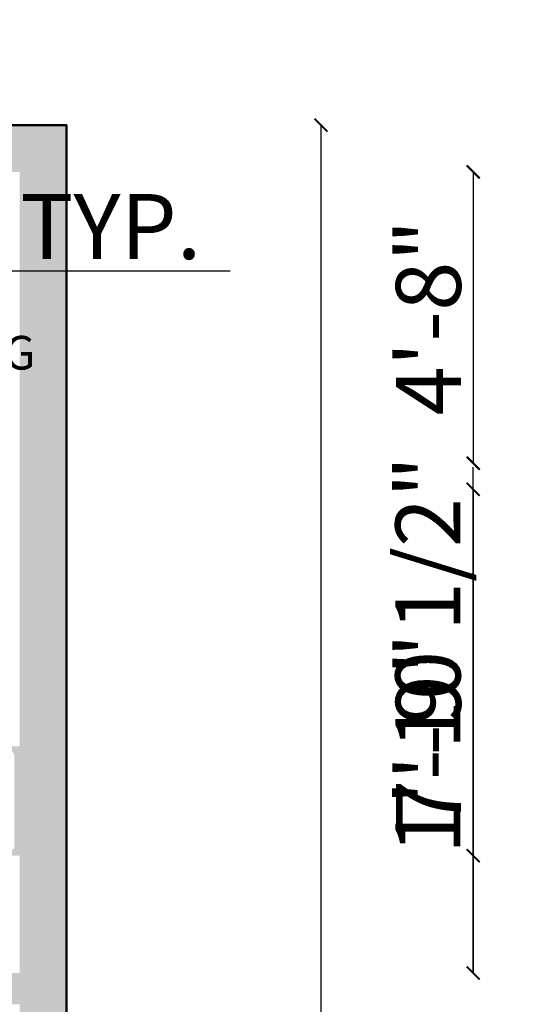
# Model space of a CAD drawing. Units: inches. Extents: x 2419 to 2878, y 1068 to 1713.
# Tile 19 of 20: x 2772 to 2870, y 1409 to 1598. Entities that reach past the tile are written whole.
import ezdxf

# ---------------------------------------------------------------- set-up
doc = ezdxf.new("R2010")
doc.units = ezdxf.units.IN
for name, color, linetype, lineweight in [('A-ANNO-DIMS', 2, 'Continuous', 18), ('A-AREA-IDEN', 7, 'Continuous', 18), ('A-FLOR-PRKG-PATT', 1, 'Continuous', 13), ('A-FURN-PATT', 254, 'Continuous', 13), ('A-WALL', 7, 'Continuous', 50)]:
    doc.layers.add(name, color=color, linetype=linetype, lineweight=lineweight)
doc.layers.add('A-FLOR-FIXT-PATT', color=254, linetype='Continuous', lineweight=13, true_color=0xd7ebd2)
doc.layers.add('A-WALL-PATT', color=18, linetype='Continuous', lineweight=13, true_color=0x000000)
doc.styles.get("Standard").update_dxf_attribs({"font": 'arial.ttf'})
doc.dimstyles.new('ISO-25', dxfattribs={"dimtxt": 12.5, "dimasz": 2.5, "dimexe": 1.25, "dimexo": 0.625, "dimtad": 1, "dimdec": 0, "dimlunit": 4, "dimtxsty": 'Standard', "dimblk": 'ARCHTICK', "dimcen": 2.5, "dimse1": 1, "dimse2": 1, "dimclrd": 4, "dimadec": 0, "dimazin": 0, "dimtfac": 1, "dimtdec": 0, "dimtmove": 0, "dimatfit": 3, "dimfxl": 1, "dimarcsym": 0})

# ---------------------------------------------------------------- blocks, each defined once
blk = doc.blocks.new('_ArchTick')
at = {"color": 0, "linetype": 'ByBlock', "const_width": 0.15}
blk.add_lwpolyline([(-0.5, -0.5), (0.5, 0.5)], dxfattribs=at)
blk = doc.blocks.new('*D16')
at = {"layer": 'A-ANNO-DIMS', "color": 0, "lineweight": -2, "transparency": 16777216}
blk.add_line((2471.51, 1623.24), (2780.51, 1623.24), dxfattribs=at)
at = {"layer": 'Defpoints', "color": 0, "transparency": 16777216}
for p in [(2780.51, 1623.24), (2471.51, 1577.81), (2780.51, 1577.81)]:
    blk.add_point(p, dxfattribs=at)
at = {"layer": 'A-ANNO-DIMS', "color": 0, "lineweight": -2, "transparency": 16777216, "xscale": 2.5, "yscale": 2.5, "zscale": 2.5, "rotation": 180}
blk.add_blockref('_ArchTick', (2471.51, 1623.24), dxfattribs=at)
at = {"layer": 'A-ANNO-DIMS', "color": 0, "lineweight": -2, "transparency": 16777216, "xscale": 2.5, "yscale": 2.5, "zscale": 2.5}
blk.add_blockref('_ArchTick', (2780.51, 1623.24), dxfattribs=at)
at = {"layer": 'A-ANNO-DIMS', "color": 0, "transparency": 16777216, "insert": (2626.01, 1630.25), "char_height": 12.5, "attachment_point": 5}
blk.add_mtext('25\'-9"', dxfattribs=at)
blk = doc.blocks.new('*D17')
at = {"layer": 'A-ANNO-DIMS', "color": 0, "lineweight": -2, "transparency": 16777216}
blk.add_line((2829.44, 1577.81), (2829.44, 1121.81), dxfattribs=at)
at = {"layer": 'Defpoints', "color": 0, "transparency": 16777216}
for p in [(2780.51, 1577.81), (2780.51, 1121.81), (2829.44, 1121.81)]:
    blk.add_point(p, dxfattribs=at)
at = {"layer": 'A-ANNO-DIMS', "color": 0, "lineweight": -2, "transparency": 16777216, "xscale": 2.5, "yscale": 2.5, "zscale": 2.5}
for p, rotation in [((2829.44, 1577.81), 90), ((2829.44, 1121.81), 270)]:
    blk.add_blockref('_ArchTick', p, dxfattribs=dict(at, rotation=rotation))
at = {"layer": 'A-ANNO-DIMS', "color": 0, "transparency": 16777216, "insert": (2822.42, 1349.81), "char_height": 12.5, "attachment_point": 5, "rotation": 90}
blk.add_mtext("38'", dxfattribs=at)
blk = doc.blocks.new('*D24')
at = {"layer": 'A-ANNO-DIMS', "color": 4, "lineweight": -2, "transparency": 16777216}
for p, q in [((2605.13, 1549.79), (2619.13, 1549.79)), ((2619.13, 1549.79), (2811.96, 1549.79))]:
    blk.add_line(p, q, dxfattribs=at)
at = {"layer": 'Defpoints', "color": 0, "transparency": 16777216}
for p in [(2605.13, 1551.89), (2619.13, 1551.89), (2619.13, 1549.79)]:
    blk.add_point(p, dxfattribs=at)
at = {"layer": 'A-ANNO-DIMS', "color": 4, "lineweight": -2, "transparency": 16777216, "xscale": 2.5, "yscale": 2.5, "zscale": 2.5, "rotation": 180}
blk.add_blockref('_ArchTick', (2605.13, 1549.79), dxfattribs=at)
at = {"layer": 'A-ANNO-DIMS', "color": 4, "lineweight": -2, "transparency": 16777216, "xscale": 2.5, "yscale": 2.5, "zscale": 2.5}
blk.add_blockref('_ArchTick', (2619.13, 1549.79), dxfattribs=at)
at = {"layer": 'A-ANNO-DIMS', "color": 0, "transparency": 16777216, "insert": (2716.8, 1556.69), "char_height": 12.5, "attachment_point": 5}
blk.add_mtext('TABLE LAMP 1\'-2" TYP.', dxfattribs=at)
blk = doc.blocks.new('*D37')
at = {"layer": 'A-ANNO-DIMS', "color": 4, "lineweight": -2, "transparency": 16777216}
for p, q in [((2736.32, 1605.01), (2771.51, 1605.01)), ((2771.51, 1605.01), (2818.42, 1605.01))]:
    blk.add_line(p, q, dxfattribs=at)
at = {"layer": 'Defpoints', "color": 0, "transparency": 16777216}
for p in [(2771.51, 1605.01), (2736.32, 1205.81), (2771.51, 1205.81)]:
    blk.add_point(p, dxfattribs=at)
at = {"layer": 'A-ANNO-DIMS', "color": 4, "lineweight": -2, "transparency": 16777216, "xscale": 2.5, "yscale": 2.5, "zscale": 2.5, "rotation": 180}
blk.add_blockref('_ArchTick', (2736.32, 1605.01), dxfattribs=at)
at = {"layer": 'A-ANNO-DIMS', "color": 4, "lineweight": -2, "transparency": 16777216, "xscale": 2.5, "yscale": 2.5, "zscale": 2.5}
blk.add_blockref('_ArchTick', (2771.51, 1605.01), dxfattribs=at)
at = {"layer": 'A-ANNO-DIMS', "color": 0, "transparency": 16777216, "insert": (2796.22, 1611.91), "char_height": 12.5, "attachment_point": 5}
blk.add_mtext('2\'-11"', dxfattribs=at)
blk = doc.blocks.new('*D49')
at = {"layer": 'A-ANNO-DIMS', "color": 4, "lineweight": -2, "transparency": 16777216}
for p, q in [((2732.27, 1605.01), (2750.85, 1605.01)), ((2750.85, 1605.01), (2815.78, 1605.01))]:
    blk.add_line(p, q, dxfattribs=at)
at = {"layer": 'Defpoints', "color": 0, "transparency": 16777216}
for p in [(2750.85, 1605.01), (2732.27, 1512.81), (2750.85, 1512.81)]:
    blk.add_point(p, dxfattribs=at)
at = {"layer": 'A-ANNO-DIMS', "color": 4, "lineweight": -2, "transparency": 16777216, "xscale": 2.5, "yscale": 2.5, "zscale": 2.5, "rotation": 180}
blk.add_blockref('_ArchTick', (2732.27, 1605.01), dxfattribs=at)
at = {"layer": 'A-ANNO-DIMS', "color": 4, "lineweight": -2, "transparency": 16777216, "xscale": 2.5, "yscale": 2.5, "zscale": 2.5}
blk.add_blockref('_ArchTick', (2750.85, 1605.01), dxfattribs=at)
at = {"layer": 'A-ANNO-DIMS', "color": 0, "transparency": 16777216, "insert": (2784.57, 1612.1), "char_height": 12.5, "attachment_point": 5}
blk.add_mtext('1\'-6 1/2"', dxfattribs=at)
blk = doc.blocks.new('*D51')
at = {"layer": 'A-ANNO-DIMS', "color": 4, "lineweight": -2, "transparency": 16777216}
for p, q in [((2738.51, 1079.92), (2771.51, 1079.92)), ((2771.51, 1079.92), (2808.71, 1079.92))]:
    blk.add_line(p, q, dxfattribs=at)
at = {"layer": 'Defpoints', "color": 0, "transparency": 16777216}
for p in [(2738.51, 1447.89), (2771.51, 1437.39), (2771.51, 1079.92)]:
    blk.add_point(p, dxfattribs=at)
at = {"layer": 'A-ANNO-DIMS', "color": 4, "lineweight": -2, "transparency": 16777216, "xscale": 2.5, "yscale": 2.5, "zscale": 2.5, "rotation": 180}
blk.add_blockref('_ArchTick', (2738.51, 1079.92), dxfattribs=at)
at = {"layer": 'A-ANNO-DIMS', "color": 4, "lineweight": -2, "transparency": 16777216, "xscale": 2.5, "yscale": 2.5, "zscale": 2.5}
blk.add_blockref('_ArchTick', (2771.51, 1079.92), dxfattribs=at)
at = {"layer": 'A-ANNO-DIMS', "color": 0, "transparency": 16777216, "insert": (2791.36, 1086.93), "char_height": 12.5, "attachment_point": 5}
blk.add_mtext('2\'-9"', dxfattribs=at)
blk = doc.blocks.new('*D52')
at = {"layer": 'A-ANNO-DIMS', "color": 4, "lineweight": -2, "transparency": 16777216}
for p, q in [((2858.71, 1437.39), (2858.71, 1512.03)), ((2858.71, 1414.81), (2858.71, 1437.39))]:
    blk.add_line(p, q, dxfattribs=at)
at = {"layer": 'Defpoints', "color": 0, "transparency": 16777216}
for p in [(2771.51, 1437.39), (2858.71, 1437.39), (2771.51, 1414.81)]:
    blk.add_point(p, dxfattribs=at)
at = {"layer": 'A-ANNO-DIMS', "color": 4, "lineweight": -2, "transparency": 16777216, "xscale": 2.5, "yscale": 2.5, "zscale": 2.5}
for p, rotation in [((2858.71, 1437.39), 90), ((2858.71, 1414.81), 270)]:
    blk.add_blockref('_ArchTick', p, dxfattribs=dict(at, rotation=rotation))
at = {"layer": 'A-ANNO-DIMS', "color": 0, "transparency": 16777216, "insert": (2851.63, 1475.96), "char_height": 12.5, "attachment_point": 5, "rotation": 90}
blk.add_mtext('1\'-10 1/2"', dxfattribs=at)
blk = doc.blocks.new('*D61')
at = {"layer": 'A-ANNO-DIMS', "color": 4, "lineweight": -2, "transparency": 16777216}
blk.add_line((2730.51, 1079.92), (2771.51, 1079.92), dxfattribs=at)
at = {"layer": 'Defpoints', "color": 0, "transparency": 16777216}
for p in [(2730.51, 1414.81), (2771.51, 1414.81), (2771.51, 1079.92)]:
    blk.add_point(p, dxfattribs=at)
at = {"layer": 'A-ANNO-DIMS', "color": 4, "lineweight": -2, "transparency": 16777216, "xscale": 2.5, "yscale": 2.5, "zscale": 2.5, "rotation": 180}
blk.add_blockref('_ArchTick', (2730.51, 1079.92), dxfattribs=at)
at = {"layer": 'A-ANNO-DIMS', "color": 4, "lineweight": -2, "transparency": 16777216, "xscale": 2.5, "yscale": 2.5, "zscale": 2.5}
blk.add_blockref('_ArchTick', (2771.51, 1079.92), dxfattribs=at)
at = {"layer": 'A-ANNO-DIMS', "color": 0, "transparency": 16777216, "insert": (2751.01, 1086.94), "char_height": 12.5, "attachment_point": 5}
blk.add_mtext('3\'-5"', dxfattribs=at)
blk = doc.blocks.new('*D62')
at = {"layer": 'A-ANNO-DIMS', "color": 4, "lineweight": -2, "transparency": 16777216}
blk.add_line((2858.71, 1507.81), (2858.71, 1414.81), dxfattribs=at)
at = {"layer": 'Defpoints', "color": 0, "transparency": 16777216}
for p in [(2771.51, 1507.81), (2771.51, 1414.81), (2858.71, 1414.81)]:
    blk.add_point(p, dxfattribs=at)
at = {"layer": 'A-ANNO-DIMS', "color": 4, "lineweight": -2, "transparency": 16777216, "xscale": 2.5, "yscale": 2.5, "zscale": 2.5}
for p, rotation in [((2858.71, 1507.81), 90), ((2858.71, 1414.81), 270)]:
    blk.add_blockref('_ArchTick', p, dxfattribs=dict(at, rotation=rotation))
at = {"layer": 'A-ANNO-DIMS', "color": 0, "transparency": 16777216, "insert": (2851.71, 1461.31), "char_height": 12.5, "attachment_point": 5, "rotation": 90}
blk.add_mtext('7\'-9"', dxfattribs=at)
blk = doc.blocks.new('*D63')
at = {"layer": 'A-ANNO-DIMS', "color": 4, "lineweight": -2, "transparency": 16777216}
blk.add_line((2858.71, 1568.81), (2858.71, 1512.81), dxfattribs=at)
at = {"layer": 'Defpoints', "color": 0, "transparency": 16777216}
for p in [(2771.51, 1568.81), (2771.51, 1512.81), (2858.71, 1512.81)]:
    blk.add_point(p, dxfattribs=at)
at = {"layer": 'A-ANNO-DIMS', "color": 4, "lineweight": -2, "transparency": 16777216, "xscale": 2.5, "yscale": 2.5, "zscale": 2.5}
for p, rotation in [((2858.71, 1568.81), 90), ((2858.71, 1512.81), 270)]:
    blk.add_blockref('_ArchTick', p, dxfattribs=dict(at, rotation=rotation))
at = {"layer": 'A-ANNO-DIMS', "color": 0, "transparency": 16777216, "insert": (2851.71, 1540.81), "char_height": 12.5, "attachment_point": 5, "rotation": 90}
blk.add_mtext('4\'-8"', dxfattribs=at)

msp = doc.modelspace()

# ---------------------------------------------------------------- hatches: boundary and pattern name
at = {"layer": 'A-FLOR-FIXT-PATT'}
h = msp.add_hatch(color=256, dxfattribs=at)
h.dxf.hatch_style = 1
h.paths.add_polyline_path([(2771.51, 1458.39), (2763.51, 1458.39), (2763.51, 1437.39), (2771.51, 1437.39)])
h.paths.add_polyline_path([(2770.51, 1456.39, 0.5), (2769.51, 1457.39), (2765.51, 1457.39, 0.5), (2764.51, 1456.39), (2764.51, 1439.39, 0.5), (2765.51, 1438.39), (2769.51, 1438.39, 0.5), (2770.51, 1439.39)], flags=16)
h.paths.add_polyline_path([(2706.38, 1408.81), (2685.38, 1408.81), (2685.38, 1400.81), (2706.38, 1400.81)])
h.paths.add_polyline_path([(2704.38, 1401.81, 0.5), (2705.38, 1402.81), (2705.38, 1406.81, 0.5), (2704.38, 1407.81), (2687.38, 1407.81, 0.5), (2686.38, 1406.81), (2686.38, 1402.81, 0.5), (2687.38, 1401.81)], flags=16)
h.paths.add_polyline_path([(2574.48, 1207.45), (2633.94, 1207.45), (2633.94, 1217.37), (2574.48, 1217.37)], flags=9)
h.paths.add_polyline_path([(2574.45, 1217.83), (2610.47, 1217.83), (2610.47, 1227.88), (2574.45, 1227.88)], flags=9)
h.paths.add_polyline_path([(2672.43, 1304.02), (2718.62, 1304.02), (2718.62, 1313.94), (2672.43, 1313.94)], flags=9)
h.paths.add_polyline_path([(2672.4, 1314.4), (2750.13, 1314.4), (2750.13, 1324.45), (2672.4, 1324.45)], flags=9)
h.paths.add_polyline_path([(2500.43, 1374.44), (2544.8, 1374.44), (2544.8, 1384.36), (2500.43, 1384.36)], flags=9)
h.paths.add_polyline_path([(2500.41, 1384.82), (2566.08, 1384.82), (2566.08, 1394.87), (2500.41, 1394.87)], flags=9)
h.paths.add_polyline_path([(2738.93, 1376.75), (2778.27, 1376.75), (2778.27, 1386.67), (2738.93, 1386.67)], flags=9)
h.paths.add_polyline_path([(2659.12, 1357.8), (2703.49, 1357.8), (2703.49, 1367.72), (2659.12, 1367.72)], flags=9)
h.paths.add_polyline_path([(2659.1, 1368.18), (2694.11, 1368.18), (2694.11, 1378.23), (2659.1, 1378.23)], flags=9)
h.paths.add_polyline_path([(2730.12, 1466.07), (2769.46, 1466.07), (2769.46, 1475.99), (2730.12, 1475.99)], flags=9)
h.paths.add_polyline_path([(2730.1, 1476.45), (2765.12, 1476.45), (2765.12, 1486.5), (2730.1, 1486.5)], flags=9)
h.paths.add_polyline_path([(2730.38, 1518.65), (2761.48, 1518.65), (2761.48, 1528.57), (2730.38, 1528.57)], flags=9)
h.paths.add_polyline_path([(2730.36, 1529.03), (2780.96, 1529.03), (2780.96, 1539.07), (2730.36, 1539.07)], flags=9)
h.paths.add_polyline_path([(2629.32, 1455.19), (2688.78, 1455.19), (2688.78, 1465.11), (2629.32, 1465.11)], flags=9)
h.paths.add_polyline_path([(2629.3, 1465.57), (2681.9, 1465.57), (2681.9, 1475.62), (2629.3, 1475.62)], flags=9)
h.paths.add_polyline_path([(2513.23, 1456.48), (2562.63, 1456.48), (2562.63, 1466.4), (2513.23, 1466.4)], flags=9)
h.paths.add_polyline_path([(2513.21, 1466.86), (2556.26, 1466.86), (2556.26, 1476.91), (2513.21, 1476.91)], flags=9)
h.paths.add_polyline_path([(2488.87, 1521.54), (2519.97, 1521.54), (2519.97, 1531.46), (2488.87, 1531.46)], flags=9)
h.paths.add_polyline_path([(2536.55, 1543.51), (2580.92, 1543.51), (2580.92, 1553.43), (2536.55, 1553.43)], flags=9)
h.paths.add_polyline_path([(2536.56, 1553.92), (2573.53, 1553.92), (2573.53, 1563.8), (2536.56, 1563.8)], flags=9)
at = {"layer": 'A-FLOR-PRKG-PATT'}
h = msp.add_hatch(color=256, dxfattribs=at)
h.dxf.hatch_style = 1
edge = h.paths.add_edge_path()
edge.add_ellipse((2561.37, 1279.45), major_axis=(3.99, 0), ratio=0.842304, start_angle=0.6466, end_angle=90)
edge.add_line((2561.37, 1282.81), (2511.57, 1282.81))
edge.add_ellipse((2511.57, 1279.45), major_axis=(3.99, 0), ratio=0.842304, start_angle=90, end_angle=179.3534)
edge.add_ellipse((10560.89, 1188.62), major_axis=(-8054.03, 0), ratio=0.8423039, start_angle=-0.646554, end_angle=-0.628237)
edge.add_ellipse((2509.23, 1276.91), major_axis=(1.69, 0), ratio=0.842304, start_angle=179.3718, end_angle=248.4648)
edge.add_ellipse((10560.33, 1188.62), major_axis=(8052.29, 0), ratio=0.8423039, start_angle=179.353446, end_angle=179.381357, ccw=False)
edge.add_ellipse((2511.01, 1279.45), major_axis=(2.25, 0), ratio=0.842304, start_angle=90, end_angle=179.3534, ccw=False)
edge.add_line((2511.01, 1281.35), (2561.94, 1281.35))
edge.add_ellipse((2561.94, 1279.45), major_axis=(-2.25, 0), ratio=0.842304, start_angle=180.6466, end_angle=270, ccw=False)
edge.add_ellipse((-5487.38, 1188.62), major_axis=(8052.29, 0), ratio=0.8423039, start_angle=0.528271, end_angle=0.646554, ccw=False)
edge.add_ellipse((2563.71, 1276.91), major_axis=(-1.69, 0), ratio=0.842304, start_angle=111.5352, end_angle=180.6282)
edge.add_ellipse((-5487.95, 1188.62), major_axis=(-8054.03, 0), ratio=0.8423039, start_angle=180.628237, end_angle=180.646554)
edge = h.paths.add_edge_path()
edge.add_ellipse((2564.91, 1261.91), major_axis=(-1.12, 0), ratio=0.842304, start_angle=180, end_angle=270)
edge.add_line((2564.91, 1262.86), (2564.43, 1262.86))
edge.add_ellipse((-5487.38, 1188.62), major_axis=(8052.29, 0), ratio=0.8423039, start_angle=0.383867, end_angle=0.528271, ccw=False)
edge.add_line((2564.65, 1242.56), (2564.91, 1242.56))
edge.add_ellipse((2564.91, 1243.51), major_axis=(-1.12, 0), ratio=0.842304, start_angle=90, end_angle=180)
edge.add_line((2566.03, 1243.51), (2566.03, 1261.91))
edge = h.paths.add_edge_path()
edge.add_ellipse((2564.91, 1174.99), major_axis=(1.12, 0), ratio=0.842304, start_angle=0, end_angle=90)
edge.add_line((2564.91, 1175.94), (2564.89, 1175.94))
edge.add_ellipse((-5487.38, 1188.62), major_axis=(8052.29, 0), ratio=0.8423039, start_angle=-0.134987, end_angle=-0.090229, ccw=False)
edge.add_ellipse((2163.34, 1170.91), major_axis=(401.54, 0), ratio=0.842304, start_angle=-2.18, end_angle=-0.1356, ccw=False)
edge.add_line((2564.47, 1155.64), (2564.91, 1155.64))
edge.add_ellipse((2564.91, 1156.59), major_axis=(-1.12, 0), ratio=0.842304, start_angle=90, end_angle=180)
edge.add_line((2566.03, 1156.59), (2566.03, 1174.99))
h.paths.add_polyline_path([(2574.48, 1207.45), (2633.94, 1207.45), (2633.94, 1217.37), (2574.48, 1217.37)], flags=9)
h.paths.add_polyline_path([(2574.45, 1217.83), (2610.47, 1217.83), (2610.47, 1227.88), (2574.45, 1227.88)], flags=9)
h.paths.add_polyline_path([(2672.43, 1304.02), (2718.62, 1304.02), (2718.62, 1313.94), (2672.43, 1313.94)], flags=9)
h.paths.add_polyline_path([(2672.4, 1314.4), (2750.13, 1314.4), (2750.13, 1324.45), (2672.4, 1324.45)], flags=9)
h.paths.add_polyline_path([(2500.43, 1374.44), (2544.8, 1374.44), (2544.8, 1384.36), (2500.43, 1384.36)], flags=9)
h.paths.add_polyline_path([(2500.41, 1384.82), (2566.08, 1384.82), (2566.08, 1394.87), (2500.41, 1394.87)], flags=9)
h.paths.add_polyline_path([(2738.93, 1376.75), (2778.27, 1376.75), (2778.27, 1386.67), (2738.93, 1386.67)], flags=9)
h.paths.add_polyline_path([(2659.12, 1357.8), (2703.49, 1357.8), (2703.49, 1367.72), (2659.12, 1367.72)], flags=9)
h.paths.add_polyline_path([(2659.1, 1368.18), (2694.11, 1368.18), (2694.11, 1378.23), (2659.1, 1378.23)], flags=9)
h.paths.add_polyline_path([(2730.12, 1466.07), (2769.46, 1466.07), (2769.46, 1475.99), (2730.12, 1475.99)], flags=9)
h.paths.add_polyline_path([(2730.1, 1476.45), (2765.12, 1476.45), (2765.12, 1486.5), (2730.1, 1486.5)], flags=9)
h.paths.add_polyline_path([(2730.38, 1518.65), (2761.48, 1518.65), (2761.48, 1528.57), (2730.38, 1528.57)], flags=9)
h.paths.add_polyline_path([(2730.36, 1529.03), (2780.96, 1529.03), (2780.96, 1539.07), (2730.36, 1539.07)], flags=9)
h.paths.add_polyline_path([(2629.32, 1455.19), (2688.78, 1455.19), (2688.78, 1465.11), (2629.32, 1465.11)], flags=9)
h.paths.add_polyline_path([(2629.3, 1465.57), (2681.9, 1465.57), (2681.9, 1475.62), (2629.3, 1475.62)], flags=9)
h.paths.add_polyline_path([(2513.23, 1456.48), (2562.63, 1456.48), (2562.63, 1466.4), (2513.23, 1466.4)], flags=9)
h.paths.add_polyline_path([(2513.21, 1466.86), (2556.26, 1466.86), (2556.26, 1476.91), (2513.21, 1476.91)], flags=9)
h.paths.add_polyline_path([(2488.87, 1521.54), (2519.97, 1521.54), (2519.97, 1531.46), (2488.87, 1531.46)], flags=9)
h.paths.add_polyline_path([(2536.55, 1543.51), (2580.92, 1543.51), (2580.92, 1553.43), (2536.55, 1553.43)], flags=9)
h.paths.add_polyline_path([(2536.56, 1553.92), (2573.53, 1553.92), (2573.53, 1563.8), (2536.56, 1563.8)], flags=9)
at = {"layer": 'A-FURN-PATT'}
h = msp.add_hatch(color=256, dxfattribs=at)
h.dxf.hatch_style = 1
h.paths.add_polyline_path([(2710.17, 1562.64), (2707.17, 1559.64), (2709.17, 1559.64, -0.414214), (2710.17, 1560.64)])
h.paths.add_polyline_path([(2711.17, 1559.64, 1), (2709.17, 1559.64, 1)])
h.paths.add_polyline_path([(2710.17, 1562.64), (2710.17, 1560.64, -0.414214), (2711.17, 1559.64), (2713.17, 1559.64)])
h.paths.add_polyline_path([(2713.17, 1559.64), (2711.17, 1559.64, -0.414214), (2710.17, 1558.64), (2710.17, 1556.64)])
h.paths.add_polyline_path([(2710.17, 1558.64, -0.414214), (2709.17, 1559.64), (2707.17, 1559.64), (2710.17, 1556.64)])
h.paths.add_polyline_path([(2613.13, 1558.89, 1), (2611.13, 1558.89, 1)])
h.paths.add_polyline_path([(2612.13, 1561.89), (2612.13, 1559.89, -0.414214), (2613.13, 1558.89), (2615.13, 1558.89)])
h.paths.add_polyline_path([(2612.13, 1559.89), (2612.13, 1561.89), (2609.13, 1558.89), (2611.13, 1558.89, -0.414214)])
h.paths.add_polyline_path([(2612.13, 1557.89, -0.414214), (2611.13, 1558.89), (2609.13, 1558.89), (2612.13, 1555.89)])
h.paths.add_polyline_path([(2574.48, 1207.45), (2633.94, 1207.45), (2633.94, 1217.37), (2574.48, 1217.37)], flags=9)
h.paths.add_polyline_path([(2574.45, 1217.83), (2610.47, 1217.83), (2610.47, 1227.88), (2574.45, 1227.88)], flags=9)
h.paths.add_polyline_path([(2672.43, 1304.02), (2718.62, 1304.02), (2718.62, 1313.94), (2672.43, 1313.94)], flags=9)
h.paths.add_polyline_path([(2672.4, 1314.4), (2750.13, 1314.4), (2750.13, 1324.45), (2672.4, 1324.45)], flags=9)
h.paths.add_polyline_path([(2500.43, 1374.44), (2544.8, 1374.44), (2544.8, 1384.36), (2500.43, 1384.36)], flags=9)
h.paths.add_polyline_path([(2500.41, 1384.82), (2566.08, 1384.82), (2566.08, 1394.87), (2500.41, 1394.87)], flags=9)
h.paths.add_polyline_path([(2738.93, 1376.75), (2778.27, 1376.75), (2778.27, 1386.67), (2738.93, 1386.67)], flags=9)
h.paths.add_polyline_path([(2659.12, 1357.8), (2703.49, 1357.8), (2703.49, 1367.72), (2659.12, 1367.72)], flags=9)
h.paths.add_polyline_path([(2659.1, 1368.18), (2694.11, 1368.18), (2694.11, 1378.23), (2659.1, 1378.23)], flags=9)
h.paths.add_polyline_path([(2730.12, 1466.07), (2769.46, 1466.07), (2769.46, 1475.99), (2730.12, 1475.99)], flags=9)
h.paths.add_polyline_path([(2730.1, 1476.45), (2765.12, 1476.45), (2765.12, 1486.5), (2730.1, 1486.5)], flags=9)
h.paths.add_polyline_path([(2730.38, 1518.65), (2761.48, 1518.65), (2761.48, 1528.57), (2730.38, 1528.57)], flags=9)
h.paths.add_polyline_path([(2730.36, 1529.03), (2780.96, 1529.03), (2780.96, 1539.07), (2730.36, 1539.07)], flags=9)
h.paths.add_polyline_path([(2629.32, 1455.19), (2688.78, 1455.19), (2688.78, 1465.11), (2629.32, 1465.11)], flags=9)
h.paths.add_polyline_path([(2629.3, 1465.57), (2681.9, 1465.57), (2681.9, 1475.62), (2629.3, 1475.62)], flags=9)
h.paths.add_polyline_path([(2513.23, 1456.48), (2562.63, 1456.48), (2562.63, 1466.4), (2513.23, 1466.4)], flags=9)
h.paths.add_polyline_path([(2513.21, 1466.86), (2556.26, 1466.86), (2556.26, 1476.91), (2513.21, 1476.91)], flags=9)
h.paths.add_polyline_path([(2488.87, 1521.54), (2519.97, 1521.54), (2519.97, 1531.46), (2488.87, 1531.46)], flags=9)
h.paths.add_polyline_path([(2536.55, 1543.51), (2580.92, 1543.51), (2580.92, 1553.43), (2536.55, 1553.43)], flags=9)
h.paths.add_polyline_path([(2536.56, 1553.92), (2573.53, 1553.92), (2573.53, 1563.8), (2536.56, 1563.8)], flags=9)
at = {"layer": 'A-WALL-PATT'}
h = msp.add_hatch(color=256, dxfattribs=at)
h.dxf.hatch_style = 1
h.paths.add_polyline_path([(2780.51, 1577.81), (2471.51, 1577.81), (2471.51, 1121.81), (2780.51, 1121.81)])
h.paths.add_polyline_path([(2480.51, 1568.81), (2771.51, 1568.81), (2771.51, 1130.81), (2480.51, 1130.81)], flags=16)
h.paths.add_polyline_path([(2528.51, 1568.81), (2528.51, 1512.81), (2594.51, 1512.81), (2594.51, 1414.81), (2596.57, 1414.81), (2596.57, 1441.61), (2597.82, 1441.61), (2597.82, 1441.58, -0.384016), (2625.03, 1414.81), (2725.51, 1414.81), (2725.51, 1567.55), (2728.3, 1567.55), (2746.89, 1567.55), (2746.89, 1566.73), (2746.87, 1566.73, -0.367216), (2730.51, 1549.09), (2730.51, 1512.81), (2750.85, 1512.81), (2750.85, 1510.03, -0.401453), (2733.08, 1491.46), (2733.08, 1491.44), (2732.27, 1491.44), (2732.27, 1507.81), (2730.51, 1507.81), (2730.51, 1408.81), (2736.51, 1408.81), (2736.51, 1349.81), (2632.51, 1349.81), (2632.51, 1408.81), (2528.51, 1408.81), (2528.51, 1414.81), (2503.97, 1414.81), (2503.97, 1494.85), (2558.38, 1494.85), (2558.38, 1507.81), (2529.96, 1507.81, -0.414214), (2530.82, 1506.96), (2530.82, 1497.26, -0.414214), (2529.96, 1496.4), (2514.56, 1496.4, -0.414214), (2513.7, 1497.26), (2513.7, 1506.96, -0.414214), (2514.56, 1507.81), (2528.51, 1507.81), (2528.51, 1512.81), (2480.51, 1512.81)], flags=0)
h.paths.add_polyline_path([(2516.26, 1507.81), (2528.26, 1507.81), (2528.26, 1505.81), (2523.42, 1505.81), (2524.07, 1504.67), (2529.39, 1504.67, -0.414214), (2529.96, 1504.1), (2529.96, 1497.83, -0.414214), (2529.39, 1497.26), (2515.13, 1497.26, -0.414214), (2514.56, 1497.83), (2514.56, 1504.1, -0.414214), (2515.13, 1504.67), (2520.69, 1504.67), (2521.34, 1505.81), (2516.26, 1505.81)], flags=0)
h.paths.add_polyline_path([(2522.02, 1505.53), (2522.82, 1507.32, -0.65506), (2522.25, 1506.06), (2522.19, 1505.93), (2522.43, 1505.53)], flags=0)
h.paths.add_polyline_path([(2522.83, 1500.97, -1), (2521.69, 1500.97, -1)], flags=0)
h.paths.add_polyline_path([(2522.55, 1500.97, -1), (2521.98, 1500.97, -1)], flags=0)
h.paths.add_polyline_path([(2482.01, 1470.63), (2499.89, 1470.63), (2499.89, 1448.27), (2482.01, 1448.27), (2482.01, 1452.74), (2481.26, 1452.74), (2481.26, 1449.76), (2480.51, 1449.76), (2480.51, 1469.14), (2481.26, 1469.14), (2481.26, 1466.16), (2482.01, 1466.16)], flags=0)
h.paths.add_polyline_path([(2488.71, 1466.16, -1), (2484.24, 1466.16, -1)], flags=0)
h.paths.add_polyline_path([(2496.17, 1466.16, -1), (2490.2, 1466.16, -1)], flags=0)
h.paths.add_polyline_path([(2487.97, 1466.16, -1), (2484.99, 1466.16, -1)], flags=0)
h.paths.add_polyline_path([(2495.42, 1466.16, -1), (2490.95, 1466.16, -1)], flags=0)
h.paths.add_polyline_path([(2487.22, 1466.16, -1), (2485.73, 1466.16, -1)], flags=0)
h.paths.add_polyline_path([(2494.68, 1466.16, -1), (2491.69, 1466.16, -1)], flags=0)
h.paths.add_polyline_path([(2499.11, 1468, -1), (2497.98, 1468, -1)], flags=0)
h.paths.add_polyline_path([(2493.93, 1466.16, -1), (2492.44, 1466.16, -1)], flags=0)
h.paths.add_polyline_path([(2499.37, 1463.71, -1), (2498.17, 1463.71, -1)], flags=0)
h.paths.add_polyline_path([(2484.24, 1461.69), (2496.17, 1461.69), (2496.17, 1457.22), (2484.24, 1457.22)], flags=0)
h.paths.add_polyline_path([(2484.99, 1460.94), (2495.42, 1460.94), (2495.42, 1457.96), (2484.99, 1457.96)], flags=0)
h.paths.add_polyline_path([(2586.88, 1510.03), (2587.69, 1510.03), (2587.69, 1491.44), (2586.88, 1491.44)], flags=0)
h.paths.add_polyline_path([(2499.26, 1459.41, -1), (2498.2, 1459.41, -1)], flags=0)
h.paths.add_polyline_path([(2489.46, 1452.74, -1), (2483.5, 1452.74, -1)], flags=0)
h.paths.add_polyline_path([(2557.3, 1408.81), (2557.3, 1413.09, -0.401453), (2584.57, 1441.58), (2584.57, 1441.61), (2585.82, 1441.61), (2585.82, 1413.09), (2585.82, 1408.81)], flags=0)
h.paths.add_polyline_path([(2488.71, 1452.74, -1), (2484.24, 1452.74, -1)], flags=0)
h.paths.add_polyline_path([(2495.42, 1452.74, -1), (2490.95, 1452.74, -1)], flags=0)
h.paths.add_polyline_path([(2487.97, 1452.74, -1), (2484.99, 1452.74, -1)], flags=0)
h.paths.add_polyline_path([(2494.68, 1452.74, -1), (2491.69, 1452.74, -1)], flags=0)
h.paths.add_polyline_path([(2487.22, 1452.74, -1), (2485.73, 1452.74, -1)], flags=0)
h.paths.add_polyline_path([(2499.18, 1454.44, -1), (2497.9, 1454.44, -1)], flags=0)
h.paths.add_polyline_path([(2493.93, 1452.74, -1), (2492.44, 1452.74, -1)], flags=0)
h.paths.add_polyline_path([(2499.3, 1450.64, -1), (2497.79, 1450.64, -1)], flags=0)
h.paths.add_polyline_path([(2619.13, 1558.89, -1), (2605.13, 1558.89, -1)], flags=0)
h.paths.add_polyline_path([(2609.13, 1558.89), (2612.13, 1561.89), (2615.13, 1558.89), (2612.13, 1555.89)], flags=0)
h.paths.add_polyline_path([(2611.13, 1558.89, -1), (2613.13, 1558.89, -1)], flags=0)
h.paths.add_polyline_path([(2633.68, 1568.81), (2693.68, 1568.81), (2693.68, 1488.81), (2633.68, 1488.81)], flags=0)
h.paths.add_polyline_path([(2641.68, 1554.41), (2641.68, 1567.61), (2662.48, 1567.61), (2662.48, 1554.41), (2664.88, 1554.41), (2664.88, 1567.61), (2685.68, 1567.61), (2685.68, 1552.41), (2680.48, 1552.41), (2693.68, 1539.21), (2678.48, 1539.21), (2678.48, 1554.41)], flags=0)
h.paths.add_polyline_path([(2637.51, 1408.81), (2731.51, 1408.81), (2731.51, 1354.81), (2637.51, 1354.81), (2637.51, 1357.98), (2635.3, 1357.98), (2635.3, 1358.79), (2637.51, 1358.79)], flags=0)
h.paths.add_polyline_path([(2717.17, 1559.64, -1), (2703.17, 1559.64, -1)], flags=0)
h.paths.add_polyline_path([(2707.17, 1559.64), (2710.17, 1562.64), (2713.17, 1559.64), (2710.17, 1556.64)], flags=0)
h.paths.add_polyline_path([(2709.17, 1559.64, -1), (2711.17, 1559.64, -1)], flags=0)
h.paths.add_polyline_path([(2685.38, 1408.81), (2706.38, 1408.81), (2706.38, 1400.81), (2699.88, 1400.81), (2701.88, 1394.81, -0.501323), (2696.92, 1375.95, -0.132891), (2694.83, 1375.95, -0.501317), (2689.88, 1394.81), (2691.88, 1400.81), (2688.88, 1400.81), (2688.88, 1399.31), (2685.88, 1399.31), (2685.88, 1400.31), (2687.88, 1400.31), (2687.88, 1400.81), (2685.38, 1400.81)], flags=0)
h.paths.add_polyline_path([(2687.38, 1407.81), (2704.38, 1407.81, -0.5), (2705.38, 1406.81), (2705.38, 1402.81, -0.5), (2704.38, 1401.81), (2687.38, 1401.81, -0.5), (2686.38, 1402.81), (2686.38, 1406.81, -0.5)], flags=0)
h.paths.add_polyline_path([(2639.51, 1205.81), (2634.51, 1205.81), (2634.51, 1293.81), (2637.51, 1293.81), (2639.51, 1293.81)], flags=0)
h.paths.add_polyline_path([(2691.88, 1394.81), (2699.88, 1394.81, -0.48008), (2697.52, 1377.29, -0.215004), (2694.23, 1377.29, -0.48008)], flags=0)
h.paths.add_polyline_path([(2757.51, 1453.89), (2763.51, 1451.89), (2763.51, 1454.89), (2762.01, 1454.89), (2762.01, 1457.89), (2763.01, 1457.89), (2763.01, 1455.89), (2763.51, 1455.89), (2763.51, 1458.39), (2771.51, 1458.39), (2771.51, 1437.39), (2763.51, 1437.39), (2763.51, 1443.89), (2757.51, 1441.89, -0.501323), (2738.65, 1446.85, -0.132891), (2738.65, 1448.94, -0.501317)], flags=0)
h.paths.add_polyline_path([(2739.99, 1449.54, -0.48008), (2757.51, 1451.89), (2757.51, 1443.89, -0.48008), (2739.99, 1446.25, -0.215004)], flags=0)
h.paths.add_polyline_path([(2765.51, 1457.39), (2769.51, 1457.39, -0.5), (2770.51, 1456.39), (2770.51, 1439.39, -0.5), (2769.51, 1438.39), (2765.51, 1438.39, -0.5), (2764.51, 1439.39), (2764.51, 1456.39, -0.5)], flags=0)
h = msp.add_hatch(color=256, dxfattribs=at)
h.dxf.hatch_style = 1
h.paths.add_polyline_path([(2771.51, 1354.81), (2736.51, 1354.81), (2736.51, 1408.81), (2771.51, 1408.81), (2771.51, 1414.81), (2625.03, 1414.81, -0.015108), (2625.09, 1413.09), (2625.09, 1408.81), (2632.51, 1408.81), (2632.51, 1376.56), (2635.3, 1376.56, -0.029838), (2637.51, 1376.43), (2637.51, 1408.81), (2731.51, 1408.81), (2731.51, 1354.81), (2637.51, 1354.81), (2637.51, 1357.98), (2635.3, 1357.98), (2632.51, 1357.98), (2632.51, 1349.81), (2771.51, 1349.81)])
h.paths.add_polyline_path([(2639.51, 1298.81), (2637.51, 1298.81), (2480.51, 1298.81), (2480.51, 1293.81), (2637.51, 1293.81), (2639.51, 1293.81)])
h.paths.add_polyline_path([(2639.51, 1293.81), (2637.51, 1293.81), (2634.51, 1293.81), (2634.51, 1244.65), (2638.79, 1244.65, -0.006332), (2639.51, 1244.64)])
h.paths.add_polyline_path([(2639.51, 1205.81), (2771.51, 1205.81), (2771.51, 1210.81), (2639.51, 1210.81), (2639.51, 1216.13), (2638.79, 1216.13), (2634.51, 1216.13), (2634.51, 1130.81), (2639.51, 1130.81)])
h.paths.add_polyline_path([(2596.57, 1413.09), (2596.57, 1414.81), (2585.82, 1414.81), (2585.82, 1413.09), (2585.82, 1408.81), (2596.57, 1408.81)])
h.paths.add_polyline_path([(2557.3, 1413.09, -0.015108), (2557.35, 1414.81), (2480.51, 1414.81), (2480.51, 1408.81), (2557.3, 1408.81)])
h.paths.add_polyline_path([(2574.48, 1207.45), (2633.94, 1207.45), (2633.94, 1217.37), (2574.48, 1217.37)], flags=9)
h.paths.add_polyline_path([(2574.45, 1217.83), (2610.47, 1217.83), (2610.47, 1227.88), (2574.45, 1227.88)], flags=9)
h.paths.add_polyline_path([(2672.43, 1304.02), (2718.62, 1304.02), (2718.62, 1313.94), (2672.43, 1313.94)], flags=9)
h.paths.add_polyline_path([(2672.4, 1314.4), (2750.13, 1314.4), (2750.13, 1324.45), (2672.4, 1324.45)], flags=9)
h.paths.add_polyline_path([(2500.43, 1374.44), (2544.8, 1374.44), (2544.8, 1384.36), (2500.43, 1384.36)], flags=9)
h.paths.add_polyline_path([(2500.41, 1384.82), (2566.08, 1384.82), (2566.08, 1394.87), (2500.41, 1394.87)], flags=9)
h.paths.add_polyline_path([(2738.93, 1376.75), (2778.27, 1376.75), (2778.27, 1386.67), (2738.93, 1386.67)], flags=9)
h.paths.add_polyline_path([(2659.12, 1357.8), (2703.49, 1357.8), (2703.49, 1367.72), (2659.12, 1367.72)], flags=25)
h.paths.add_polyline_path([(2659.1, 1368.18), (2694.11, 1368.18), (2694.11, 1378.23), (2659.1, 1378.23)], flags=25)
h.paths.add_polyline_path([(2730.12, 1466.07), (2769.46, 1466.07), (2769.46, 1475.99), (2730.12, 1475.99)], flags=9)
h.paths.add_polyline_path([(2730.1, 1476.45), (2765.12, 1476.45), (2765.12, 1486.5), (2730.1, 1486.5)], flags=9)
h.paths.add_polyline_path([(2730.38, 1518.65), (2761.48, 1518.65), (2761.48, 1528.57), (2730.38, 1528.57)], flags=9)
h.paths.add_polyline_path([(2730.36, 1529.03), (2780.96, 1529.03), (2780.96, 1539.07), (2730.36, 1539.07)], flags=9)
h.paths.add_polyline_path([(2629.32, 1455.19), (2688.78, 1455.19), (2688.78, 1465.11), (2629.32, 1465.11)], flags=9)
h.paths.add_polyline_path([(2629.3, 1465.57), (2681.9, 1465.57), (2681.9, 1475.62), (2629.3, 1475.62)], flags=9)
h.paths.add_polyline_path([(2513.23, 1456.48), (2562.63, 1456.48), (2562.63, 1466.4), (2513.23, 1466.4)], flags=9)
h.paths.add_polyline_path([(2513.21, 1466.86), (2556.26, 1466.86), (2556.26, 1476.91), (2513.21, 1476.91)], flags=9)
h.paths.add_polyline_path([(2488.87, 1521.54), (2519.97, 1521.54), (2519.97, 1531.46), (2488.87, 1531.46)], flags=9)
h.paths.add_polyline_path([(2536.55, 1543.51), (2580.92, 1543.51), (2580.92, 1553.43), (2536.55, 1553.43)], flags=9)
h.paths.add_polyline_path([(2536.56, 1553.92), (2573.53, 1553.92), (2573.53, 1563.8), (2536.56, 1563.8)], flags=9)

# ---------------------------------------------------------------- linework, layer by layer
at = {"layer": 'A-WALL'}
msp.add_lwpolyline([(2471.51, 1577.81), (2780.51, 1577.81), (2780.51, 1121.81), (2471.51, 1121.81)], close=True, dxfattribs=at)

# ---------------------------------------------------------------- texts
at = {"layer": 'A-AREA-IDEN'}
msp.add_text('DRESSING', height=6.475, dxfattribs=at).set_placement((2732.04, 1530.81))

# ---------------------------------------------------------------- dimensions: what is measured, and where the dimension line sits
at = {"layer": 'A-ANNO-DIMS'}
for base, p1, p2, override, picture, middle in [((2780.51, 1623.24), (2471.51, 1577.81), (2780.51, 1577.81), {"dimclrd": 0, "dimclre": 0, "dimclrt": 0}, '*D16', (2626.01, 1630.25)), ((2750.85, 1605.01), (2732.27, 1512.81), (2750.85, 1512.81), {"dimdec": 1, "dimlfac": 1, "dimrnd": 0, "dimzin": 1, "dimdsep": 46, "dimlunit": 4, "dimfrac": 2}, '*D49', (2784.57, 1612.1)), ((2771.51, 1605.01), (2736.32, 1205.81), (2771.51, 1205.81), {"dimdec": 1, "dimlfac": 1, "dimrnd": 0, "dimzin": 1, "dimdsep": 46, "dimlunit": 4, "dimfrac": 2}, '*D37', (2796.22, 1611.91)), ((2771.51, 1079.92), (2738.51, 1447.89), (2771.51, 1437.39), {"dimdec": 1, "dimlfac": 1, "dimrnd": 0, "dimzin": 1, "dimdsep": 46, "dimlunit": 4, "dimfrac": 2}, '*D51', (2791.36, 1086.93)), ((2771.51, 1079.92), (2730.51, 1414.81), (2771.51, 1414.81), {"dimdec": 1, "dimlfac": 1, "dimrnd": 0, "dimzin": 1, "dimdsep": 46, "dimlunit": 4, "dimfrac": 2}, '*D61', (2751.01, 1086.94))]:
    dim = msp.add_linear_dim(base=base, p1=p1, p2=p2, dimstyle='ISO-25', override=override, dxfattribs=at)
    dim.commit()
    dim.dimension.update_dxf_attribs({"geometry": picture, "text_midpoint": middle})
dim = msp.add_linear_dim(base=(2619.13, 1549.79), p1=(2605.13, 1551.89), p2=(2619.13, 1551.89), text='TABLE LAMP <> TYP.', dimstyle='ISO-25', override={"dimdec": 1, "dimlfac": 1, "dimrnd": 0, "dimzin": 1, "dimdsep": 46, "dimlunit": 4, "dimfrac": 2}, dxfattribs=at)
dim.commit()
dim.dimension.update_dxf_attribs({"geometry": '*D24', "text_midpoint": (2716.8, 1556.69)})
for base, p1, p2, override, picture, middle in [((2829.44, 1121.81), (2780.51, 1577.81), (2780.51, 1121.81), {"dimclrd": 0, "dimclre": 0, "dimclrt": 0}, '*D17', (2822.42, 1349.81)), ((2858.71, 1512.81), (2771.51, 1568.81), (2771.51, 1512.81), {"dimdec": 1, "dimlfac": 1, "dimrnd": 0, "dimzin": 1, "dimdsep": 46, "dimlunit": 4, "dimfrac": 2}, '*D63', (2851.71, 1540.81)), ((2858.71, 1437.39), (2771.51, 1414.81), (2771.51, 1437.39), {"dimdec": 1, "dimlfac": 1, "dimrnd": 0, "dimzin": 1, "dimdsep": 46, "dimlunit": 4, "dimfrac": 2}, '*D52', (2851.63, 1475.96)), ((2858.71, 1414.81), (2771.51, 1507.81), (2771.51, 1414.81), {"dimdec": 1, "dimlfac": 1, "dimrnd": 0, "dimzin": 1, "dimdsep": 46, "dimlunit": 4, "dimfrac": 2}, '*D62', (2851.71, 1461.31))]:
    dim = msp.add_linear_dim(base=base, p1=p1, p2=p2, angle=90, dimstyle='ISO-25', override=override, dxfattribs=at)
    dim.commit()
    dim.dimension.update_dxf_attribs({"geometry": picture, "text_midpoint": middle})

doc.saveas('drawing.dxf')
